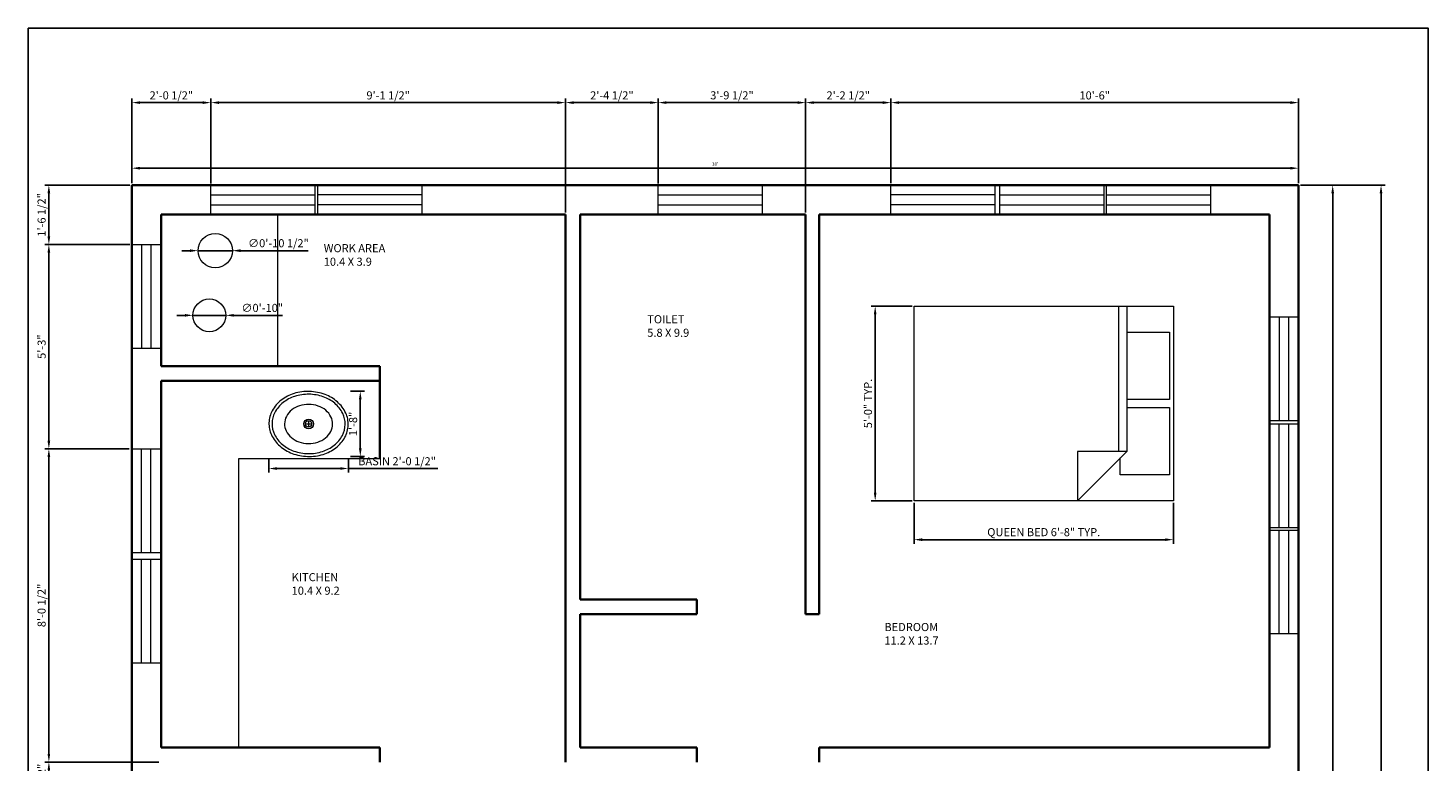
# Model space of a CAD drawing. Units: inches. Extents: x 185 to 617, y 27 to 601.
# Tile 2 of 2: x 185 to 617, y 374 to 601. Entities that reach past the tile are written whole.
import ezdxf

# ---------------------------------------------------------------- set-up
doc = ezdxf.new("R2010")
doc.units = ezdxf.units.IN
for name, color, linetype, lineweight in [('A-ANNO-DIMS', 2, 'Continuous', 18), ('A-ANNO-TTLB', 7, 'Continuous', 25), ('A-AREA-IDEN', 7, 'Continuous', 18), ('A-FLOR-FIXT', 9, 'Continuous', 18), ('A-FURN', 8, 'Continuous', 18), ('A-GLAZ', 4, 'Continuous', 18), ('A-WALL', 7, 'Continuous', 35)]:
    doc.layers.add(name, color=color, linetype=linetype, lineweight=lineweight)
doc.styles.get("Standard").update_dxf_attribs({"font": 'arial.ttf'})
doc.dimstyles.new('ISO-25', dxfattribs={"dimtxt": 2.5, "dimasz": 2.5, "dimexe": 1.25, "dimexo": 0.625, "dimtad": 1, "dimtxsty": 'Standard', "dimcen": 2.5, "dimadec": 0, "dimazin": 0, "dimtfac": 1, "dimtmove": 0, "dimatfit": 3, "dimfxl": 1, "dimarcsym": 0})

# ---------------------------------------------------------------- blocks, each defined once
blk = doc.blocks.new('Sink - Oval top')
for p, q in [((-1, 0), (1, 0)), ((0, 1), (0, -1))]:
    blk.add_line(p, q)
for points in [[(-12.23, 0.39, 0.117634), (-11.46, -3.36, 0.104469), (-8.88, -6.8, 0.090016), (-5.08, -9.07, 0.08192), (-0.32, -10.02, 0.08192), (4.49, -9.38, 0.090016), (8.42, -7.36, 0.104469), (11.22, -4.09, 0.117634), (12.23, -0.39, 0.117634), (11.46, 3.36, 0.104469), (8.88, 6.8, 0.090016), (5.08, 9.07, 0.08192), (0.32, 10.02, 0.08192), (-4.49, 9.38, 0.090016), (-8.42, 7.36, 0.104469), (-11.22, 4.09, 0.117634)], [(-11.29, 0.16, 0.118622), (-10.52, -3.25, 0.104678), (-8.07, -6.36, 0.089562), (-4.54, -8.37, 0.081185), (-0.13, -9.15, 0.081185), (4.3, -8.49, 0.089562), (7.89, -6.58, 0.104678), (10.42, -3.55, 0.118622), (11.29, -0.16, 0.118622), (10.52, 3.25, 0.104678), (8.07, 6.36, 0.089562), (4.54, 8.37, 0.081185), (0.13, 9.15, 0.081185), (-4.3, 8.49, 0.089562), (-7.89, 6.58, 0.104678), (-10.42, 3.55, 0.118622)], [(-7.42, 0.08, 0.118283), (-6.91, -2.17, 0.104607), (-5.29, -4.21, 0.089718), (-2.97, -5.53, 0.081436), (-0.07, -6.04, 0.081436), (2.84, -5.59, 0.089718), (5.2, -4.33, 0.104607), (6.86, -2.32, 0.118283), (7.42, -0.08, 0.118283), (6.91, 2.17, 0.104607), (5.29, 4.21, 0.089718), (2.97, 5.53, 0.081436), (0.07, 6.04, 0.081436), (-2.84, 5.59, 0.089718), (-5.2, 4.33, 0.104607), (-6.86, 2.32, 0.118283)]]:
    blk.add_lwpolyline(points, format="xyb", close=True)
for radius in [1.5, 1]:
    blk.add_circle((0, 0), radius)
blk = doc.blocks.new('Bed - Queen')
for p, q in [((0, -80.00003), (0, 0)), ((0, 0), (59.99999, 0)), ((59.99999, 0), (59.99999, -80.00003)), ((7.99999, -1.2), (28.79998, -1.2)), ((7.99999, -14.4), (7.99999, -1.2)), ((28.79998, -1.2), (28.79998, -14.4)), ((31.19999, -1.2), (51.99999, -1.2)), ((31.19999, -14.4), (31.19999, -1.2)), ((51.99999, -1.2), (51.99999, -16.4)), ((0, -14.4), (44.8, -14.4)), ((44.8, -16.8), (0, -16.8)), ((59.99999, -29.6), (44.8, -14.4)), ((44.8, -14.4), (44.8, -29.6)), ((51.99999, -16.4), (46.79936, -16.4)), ((44.8, -29.6), (59.99999, -29.6)), ((59.99999, -80.00003), (0, -80.00003))]:
    blk.add_line(p, q)
blk = doc.blocks.new('*D6')
at = {"layer": 'A-ANNO-DIMS', "color": 0, "lineweight": -2, "transparency": 16777216}
for p, q in [((217.11, 552.94), (217.11, 558.81)), ((219.61, 557.56), (574.61, 557.56)), ((577.11, 552.94), (577.11, 558.81))]:
    blk.add_line(p, q, dxfattribs=at)
at = {"layer": 'A-ANNO-DIMS', "color": 0, "transparency": 16777216}
for points in [[(219.61, 557.98), (219.61, 557.15), (217.11, 557.56)], [(574.61, 557.98), (574.61, 557.15), (577.11, 557.56)]]:
    blk.add_solid(points, dxfattribs=at)
at = {"layer": 'Defpoints', "color": 0, "transparency": 16777216}
for p in [(577.11, 557.56), (217.11, 552.31), (577.11, 552.31)]:
    blk.add_point(p, dxfattribs=at)
at = {"layer": 'A-ANNO-DIMS', "color": 0, "transparency": 16777216, "insert": (397.11, 558.7), "char_height": 1, "attachment_point": 5}
blk.add_mtext("30'", dxfattribs=at)
blk = doc.blocks.new('*D7')
at = {"layer": 'A-ANNO-DIMS', "color": 0, "lineweight": -2, "transparency": 16777216}
for p, q in [((577.73, 552.31), (588.89, 552.31)), ((587.64, 549.81), (587.64, 74.81)), ((577.73, 72.31), (588.89, 72.31))]:
    blk.add_line(p, q, dxfattribs=at)
at = {"layer": 'A-ANNO-DIMS', "color": 0, "transparency": 16777216}
for points in [[(587.22, 549.81), (588.05, 549.81), (587.64, 552.31)], [(587.22, 74.81), (588.05, 74.81), (587.64, 72.31)]]:
    blk.add_solid(points, dxfattribs=at)
at = {"layer": 'Defpoints', "color": 0, "transparency": 16777216}
for p in [(577.11, 552.31), (577.11, 72.31), (587.64, 72.31)]:
    blk.add_point(p, dxfattribs=at)
at = {"layer": 'A-ANNO-DIMS', "color": 0, "transparency": 16777216, "insert": (586.5, 312.31), "char_height": 1, "attachment_point": 5, "rotation": 90}
blk.add_mtext("40'", dxfattribs=at)
blk = doc.blocks.new('WIN-32IN-EXT')
for p, q in [((0, 0), (0, 32.06)), ((0, 32.06), (9, 32.06)), ((3, 32.06), (3, 0)), ((6, 0), (6, 32.06)), ((9, 32.06), (9, 0)), ((9, 0), (0, 0))]:
    blk.add_line(p, q)
blk = doc.blocks.new('*D19')
at = {"layer": 'A-ANNO-DIMS', "color": 0, "lineweight": -2, "transparency": 16777216}
for p, q in [((458.47, 454.36), (458.47, 441.73)), ((538.47, 454.36), (538.47, 441.73)), ((460.97, 442.98), (535.97, 442.98))]:
    blk.add_line(p, q, dxfattribs=at)
at = {"layer": 'A-ANNO-DIMS', "color": 0, "transparency": 16777216}
for points in [[(460.97, 443.4), (460.97, 442.57), (458.47, 442.98)], [(535.97, 443.4), (535.97, 442.57), (538.47, 442.98)]]:
    blk.add_solid(points, dxfattribs=at)
at = {"layer": 'Defpoints', "color": 0, "transparency": 16777216}
for p in [(458.47, 454.98), (538.47, 454.98), (538.47, 442.98)]:
    blk.add_point(p, dxfattribs=at)
at = {"layer": 'A-ANNO-DIMS', "color": 0, "transparency": 16777216, "insert": (498.47, 444.98), "char_height": 2.5, "attachment_point": 5}
blk.add_mtext('QUEEN BED 6\'-8" TYP.', dxfattribs=at)
blk = doc.blocks.new('*D20')
at = {"layer": 'A-ANNO-DIMS', "color": 0, "lineweight": -2, "transparency": 16777216}
for p, q in [((457.84, 514.98), (445.22, 514.98)), ((446.47, 512.48), (446.47, 457.48)), ((457.84, 454.98), (445.22, 454.98))]:
    blk.add_line(p, q, dxfattribs=at)
at = {"layer": 'A-ANNO-DIMS', "color": 0, "transparency": 16777216}
for points in [[(446.05, 512.48), (446.88, 512.48), (446.47, 514.98)], [(446.05, 457.48), (446.88, 457.48), (446.47, 454.98)]]:
    blk.add_solid(points, dxfattribs=at)
at = {"layer": 'Defpoints', "color": 0, "transparency": 16777216}
for p in [(458.47, 514.98), (446.47, 454.98), (458.47, 454.98)]:
    blk.add_point(p, dxfattribs=at)
at = {"layer": 'A-ANNO-DIMS', "color": 0, "transparency": 16777216, "insert": (444.57, 484.98), "char_height": 2.5, "attachment_point": 5, "rotation": 90}
blk.add_mtext('5\'-0" TYP.', dxfattribs=at)
blk = doc.blocks.new('*D23')
at = {"layer": 'A-ANNO-DIMS', "color": 0, "lineweight": -2, "transparency": 16777216}
for p, q in [((259.36, 467.99), (259.36, 463.68)), ((283.91, 467.99), (283.91, 463.68)), ((261.86, 464.93), (281.41, 464.93)), ((283.91, 464.93), (311.47, 464.93))]:
    blk.add_line(p, q, dxfattribs=at)
at = {"layer": 'A-ANNO-DIMS', "color": 0, "transparency": 16777216}
for points in [[(261.86, 465.35), (261.86, 464.52), (259.36, 464.93)], [(281.41, 465.35), (281.41, 464.52), (283.91, 464.93)]]:
    blk.add_solid(points, dxfattribs=at)
at = {"layer": 'Defpoints', "color": 0, "transparency": 16777216}
for p in [(259.36, 468.62), (283.91, 468.62), (283.91, 464.93)]:
    blk.add_point(p, dxfattribs=at)
at = {"layer": 'A-ANNO-DIMS', "color": 0, "transparency": 16777216, "insert": (298.94, 466.85), "char_height": 2.5, "attachment_point": 5}
blk.add_mtext('BASIN 2\'-0 1/2"', dxfattribs=at)
blk = doc.blocks.new('*D24')
at = {"layer": 'A-ANNO-DIMS', "color": 0, "lineweight": -2, "transparency": 16777216}
for p, q in [((284.54, 488.75), (288.84, 488.75)), ((287.59, 471.12), (287.59, 486.25)), ((284.54, 468.62), (288.84, 468.62))]:
    blk.add_line(p, q, dxfattribs=at)
at = {"layer": 'A-ANNO-DIMS', "color": 0, "transparency": 16777216}
for points in [[(287.18, 486.25), (288.01, 486.25), (287.59, 488.75)], [(287.18, 471.12), (288.01, 471.12), (287.59, 468.62)]]:
    blk.add_solid(points, dxfattribs=at)
at = {"layer": 'Defpoints', "color": 0, "transparency": 16777216}
for p in [(283.91, 488.75), (287.59, 488.75), (283.91, 468.62)]:
    blk.add_point(p, dxfattribs=at)
at = {"layer": 'A-ANNO-DIMS', "color": 0, "transparency": 16777216, "insert": (285.69, 478.68), "char_height": 2.5, "attachment_point": 5, "rotation": 90}
blk.add_mtext('1\'-8"', dxfattribs=at)
blk = doc.blocks.new('*D25')
at = {"layer": 'A-ANNO-DIMS', "color": 0, "lineweight": -2, "transparency": 16777216}
for p, q in [((577.73, 552.31), (603.81, 552.31)), ((602.56, 63.07), (602.56, 549.81)), ((429.78, 60.57), (603.81, 60.57))]:
    blk.add_line(p, q, dxfattribs=at)
at = {"layer": 'A-ANNO-DIMS', "color": 0, "transparency": 16777216}
for points in [[(602.14, 549.81), (602.97, 549.81), (602.56, 552.31)], [(602.14, 63.07), (602.97, 63.07), (602.56, 60.57)]]:
    blk.add_solid(points, dxfattribs=at)
at = {"layer": 'Defpoints', "color": 0, "transparency": 16777216}
for p in [(577.11, 552.31), (602.56, 552.31), (429.16, 60.57)]:
    blk.add_point(p, dxfattribs=at)
at = {"layer": 'A-ANNO-DIMS', "color": 0, "transparency": 16777216, "insert": (600.64, 306.44), "char_height": 2.5, "attachment_point": 5, "rotation": 90}
blk.add_mtext('40\'-11 1/2"', dxfattribs=at)
blk = doc.blocks.new('*D31')
at = {"layer": 'A-ANNO-DIMS', "color": 0, "lineweight": -2, "transparency": 16777216}
for p, q in [((217.11, 552.94), (217.11, 579.04)), ((241.48, 552.86), (241.48, 579.04)), ((219.61, 577.79), (238.98, 577.79))]:
    blk.add_line(p, q, dxfattribs=at)
at = {"layer": 'A-ANNO-DIMS', "color": 0, "transparency": 16777216}
for points in [[(219.61, 578.2), (219.61, 577.37), (217.11, 577.79)], [(238.98, 578.2), (238.98, 577.37), (241.48, 577.79)]]:
    blk.add_solid(points, dxfattribs=at)
at = {"layer": 'Defpoints', "color": 0, "transparency": 16777216}
for p in [(241.48, 577.79), (217.11, 552.31), (241.48, 552.23)]:
    blk.add_point(p, dxfattribs=at)
at = {"layer": 'A-ANNO-DIMS', "color": 0, "transparency": 16777216, "insert": (229.29, 579.7), "char_height": 2.5, "attachment_point": 5}
blk.add_mtext('2\'-0 1/2"', dxfattribs=at)
blk = doc.blocks.new('*D32')
at = {"layer": 'A-ANNO-DIMS', "color": 0, "lineweight": -2, "transparency": 16777216}
for p, q in [((241.48, 552.86), (241.48, 579.04)), ((350.91, 543.94), (350.91, 579.04)), ((243.98, 577.79), (348.41, 577.79))]:
    blk.add_line(p, q, dxfattribs=at)
at = {"layer": 'A-ANNO-DIMS', "color": 0, "transparency": 16777216}
for points in [[(243.98, 578.2), (243.98, 577.37), (241.48, 577.79)], [(348.41, 578.2), (348.41, 577.37), (350.91, 577.79)]]:
    blk.add_solid(points, dxfattribs=at)
at = {"layer": 'Defpoints', "color": 0, "transparency": 16777216}
for p in [(350.91, 577.79), (241.48, 552.23), (350.91, 543.31)]:
    blk.add_point(p, dxfattribs=at)
at = {"layer": 'A-ANNO-DIMS', "color": 0, "transparency": 16777216, "insert": (296.19, 579.7), "char_height": 2.5, "attachment_point": 5}
blk.add_mtext('9\'-1 1/2"', dxfattribs=at)
blk = doc.blocks.new('*D33')
at = {"layer": 'A-ANNO-DIMS', "color": 0, "lineweight": -2, "transparency": 16777216}
for p, q in [((350.91, 543.94), (350.91, 579.04)), ((379.55, 552.85), (379.55, 579.04)), ((353.41, 577.79), (377.05, 577.79))]:
    blk.add_line(p, q, dxfattribs=at)
at = {"layer": 'A-ANNO-DIMS', "color": 0, "transparency": 16777216}
for points in [[(353.41, 578.2), (353.41, 577.37), (350.91, 577.79)], [(377.05, 578.2), (377.05, 577.37), (379.55, 577.79)]]:
    blk.add_solid(points, dxfattribs=at)
at = {"layer": 'Defpoints', "color": 0, "transparency": 16777216}
for p in [(379.55, 577.79), (379.55, 552.22), (350.91, 543.31)]:
    blk.add_point(p, dxfattribs=at)
at = {"layer": 'A-ANNO-DIMS', "color": 0, "transparency": 16777216, "insert": (365.23, 579.7), "char_height": 2.5, "attachment_point": 5}
blk.add_mtext('2\'-4 1/2"', dxfattribs=at)
blk = doc.blocks.new('*D34')
at = {"layer": 'A-ANNO-DIMS', "color": 0, "lineweight": -2, "transparency": 16777216}
for p, q in [((379.55, 552.85), (379.55, 579.04)), ((425.01, 543.94), (425.01, 579.04)), ((382.05, 577.79), (422.51, 577.79))]:
    blk.add_line(p, q, dxfattribs=at)
at = {"layer": 'A-ANNO-DIMS', "color": 0, "transparency": 16777216}
for points in [[(382.05, 578.2), (382.05, 577.37), (379.55, 577.79)], [(422.51, 578.2), (422.51, 577.37), (425.01, 577.79)]]:
    blk.add_solid(points, dxfattribs=at)
at = {"layer": 'Defpoints', "color": 0, "transparency": 16777216}
for p in [(425.01, 577.79), (379.55, 552.22), (425.01, 543.31)]:
    blk.add_point(p, dxfattribs=at)
at = {"layer": 'A-ANNO-DIMS', "color": 0, "transparency": 16777216, "insert": (402.28, 579.71), "char_height": 2.5, "attachment_point": 5}
blk.add_mtext('3\'-9 1/2"', dxfattribs=at)
blk = doc.blocks.new('*D35')
at = {"layer": 'A-ANNO-DIMS', "color": 0, "lineweight": -2, "transparency": 16777216}
for p, q in [((425.01, 543.94), (425.01, 579.04)), ((451.32, 552.96), (451.32, 579.04)), ((427.51, 577.79), (448.82, 577.79))]:
    blk.add_line(p, q, dxfattribs=at)
at = {"layer": 'A-ANNO-DIMS', "color": 0, "transparency": 16777216}
for points in [[(427.51, 578.2), (427.51, 577.37), (425.01, 577.79)], [(448.82, 578.2), (448.82, 577.37), (451.32, 577.79)]]:
    blk.add_solid(points, dxfattribs=at)
at = {"layer": 'Defpoints', "color": 0, "transparency": 16777216}
for p in [(451.32, 577.79), (451.32, 552.34), (425.01, 543.31)]:
    blk.add_point(p, dxfattribs=at)
at = {"layer": 'A-ANNO-DIMS', "color": 0, "transparency": 16777216, "insert": (438.16, 579.7), "char_height": 2.5, "attachment_point": 5}
blk.add_mtext('2\'-2 1/2"', dxfattribs=at)
blk = doc.blocks.new('*D36')
at = {"layer": 'A-ANNO-DIMS', "color": 0, "lineweight": -2, "transparency": 16777216}
for p, q in [((451.32, 552.96), (451.32, 579.04)), ((577.11, 552.94), (577.11, 579.04)), ((453.82, 577.79), (574.61, 577.79))]:
    blk.add_line(p, q, dxfattribs=at)
at = {"layer": 'A-ANNO-DIMS', "color": 0, "transparency": 16777216}
for points in [[(453.82, 578.2), (453.82, 577.37), (451.32, 577.79)], [(574.61, 578.2), (574.61, 577.37), (577.11, 577.79)]]:
    blk.add_solid(points, dxfattribs=at)
at = {"layer": 'Defpoints', "color": 0, "transparency": 16777216}
for p in [(577.11, 577.79), (451.32, 552.34), (577.11, 552.31)]:
    blk.add_point(p, dxfattribs=at)
at = {"layer": 'A-ANNO-DIMS', "color": 0, "transparency": 16777216, "insert": (514.21, 579.69), "char_height": 2.5, "attachment_point": 5}
blk.add_mtext('10\'-6"', dxfattribs=at)
blk = doc.blocks.new('*D37')
at = {"layer": 'A-ANNO-DIMS', "color": 0, "lineweight": -2, "transparency": 16777216}
for p, q in [((216.48, 552.31), (190.25, 552.31)), ((191.5, 549.81), (191.5, 536.5)), ((216.46, 534), (190.25, 534))]:
    blk.add_line(p, q, dxfattribs=at)
at = {"layer": 'A-ANNO-DIMS', "color": 0, "transparency": 16777216}
for points in [[(191.08, 549.81), (191.91, 549.81), (191.5, 552.31)], [(191.08, 536.5), (191.91, 536.5), (191.5, 534)]]:
    blk.add_solid(points, dxfattribs=at)
at = {"layer": 'Defpoints', "color": 0, "transparency": 16777216}
for p in [(217.11, 552.31), (191.5, 534), (217.08, 534)]:
    blk.add_point(p, dxfattribs=at)
at = {"layer": 'A-ANNO-DIMS', "color": 0, "transparency": 16777216, "insert": (189.58, 543.16), "char_height": 2.5, "attachment_point": 5, "rotation": 90}
blk.add_mtext('1\'-6 1/2"', dxfattribs=at)
blk = doc.blocks.new('*D38')
at = {"layer": 'A-ANNO-DIMS', "color": 0, "lineweight": -2, "transparency": 16777216}
for p, q in [((216.46, 534), (190.25, 534)), ((191.5, 531.5), (191.5, 473.52)), ((216.32, 471.02), (190.25, 471.02))]:
    blk.add_line(p, q, dxfattribs=at)
at = {"layer": 'A-ANNO-DIMS', "color": 0, "transparency": 16777216}
for points in [[(191.08, 531.5), (191.91, 531.5), (191.5, 534)], [(191.08, 473.52), (191.91, 473.52), (191.5, 471.02)]]:
    blk.add_solid(points, dxfattribs=at)
at = {"layer": 'Defpoints', "color": 0, "transparency": 16777216}
for p in [(217.08, 534), (191.5, 471.02), (216.95, 471.02)]:
    blk.add_point(p, dxfattribs=at)
at = {"layer": 'A-ANNO-DIMS', "color": 0, "transparency": 16777216, "insert": (189.59, 502.51), "char_height": 2.5, "attachment_point": 5, "rotation": 90}
blk.add_mtext('5\'-3"', dxfattribs=at)
blk = doc.blocks.new('*D39')
at = {"layer": 'A-ANNO-DIMS', "color": 0, "lineweight": -2, "transparency": 16777216}
for p, q in [((216.32, 471.02), (190.25, 471.02)), ((191.5, 468.52), (191.5, 376.91)), ((225.48, 374.41), (190.25, 374.41))]:
    blk.add_line(p, q, dxfattribs=at)
at = {"layer": 'A-ANNO-DIMS', "color": 0, "transparency": 16777216}
for points in [[(191.08, 468.52), (191.91, 468.52), (191.5, 471.02)], [(191.08, 376.91), (191.91, 376.91), (191.5, 374.41)]]:
    blk.add_solid(points, dxfattribs=at)
at = {"layer": 'Defpoints', "color": 0, "transparency": 16777216}
for p in [(216.95, 471.02), (191.5, 374.41), (226.11, 374.41)]:
    blk.add_point(p, dxfattribs=at)
at = {"layer": 'A-ANNO-DIMS', "color": 0, "transparency": 16777216, "insert": (189.58, 422.71), "char_height": 2.5, "attachment_point": 5, "rotation": 90}
blk.add_mtext('8\'-0 1/2"', dxfattribs=at)
blk = doc.blocks.new('*D40')
at = {"layer": 'A-ANNO-DIMS', "color": 0, "lineweight": -2, "transparency": 16777216}
for p, q in [((225.48, 374.41), (190.25, 374.41)), ((191.5, 371.91), (191.5, 362.42)), ((216.42, 359.92), (190.25, 359.92))]:
    blk.add_line(p, q, dxfattribs=at)
at = {"layer": 'A-ANNO-DIMS', "color": 0, "transparency": 16777216}
for points in [[(191.08, 371.91), (191.91, 371.91), (191.5, 374.41)], [(191.08, 362.42), (191.91, 362.42), (191.5, 359.92)]]:
    blk.add_solid(points, dxfattribs=at)
at = {"layer": 'Defpoints', "color": 0, "transparency": 16777216}
for p in [(226.11, 374.41), (191.5, 359.92), (217.05, 359.92)]:
    blk.add_point(p, dxfattribs=at)
at = {"layer": 'A-ANNO-DIMS', "color": 0, "transparency": 16777216, "insert": (189.58, 367.17), "char_height": 2.5, "attachment_point": 5, "rotation": 90}
blk.add_mtext('1\'-2 1/2"', dxfattribs=at)
blk = doc.blocks.new('*D44')
at = {"layer": 'A-ANNO-DIMS', "color": 0, "lineweight": -2, "transparency": 16777216}
for p, q in [((235.02, 532.12), (232.52, 532.12)), ((237.52, 532.12), (248.14, 532.12)), ((271.52, 532.12), (250.64, 532.12))]:
    blk.add_line(p, q, dxfattribs=at)
at = {"layer": 'A-ANNO-DIMS', "color": 0, "transparency": 16777216}
for points in [[(235.02, 532.54), (235.02, 531.71), (237.52, 532.12)], [(250.64, 532.54), (250.64, 531.71), (248.14, 532.12)]]:
    blk.add_solid(points, dxfattribs=at)
at = {"layer": 'Defpoints', "color": 0, "transparency": 16777216}
for p in [(237.52, 532.12), (248.14, 532.12)]:
    blk.add_point(p, dxfattribs=at)
at = {"layer": 'A-ANNO-DIMS', "color": 0, "transparency": 16777216, "insert": (262.33, 534.1), "char_height": 2.5, "attachment_point": 5, "rotation": 0.0037}
blk.add_mtext('∅0\'-10 1/2"', dxfattribs=at)
blk = doc.blocks.new('*D45')
at = {"layer": 'A-ANNO-DIMS', "color": 0, "lineweight": -2, "transparency": 16777216}
for p, q in [((233.46, 512.17), (230.96, 512.17)), ((235.96, 512.17), (246.07, 512.17)), ((263.62, 512.17), (248.57, 512.17))]:
    blk.add_line(p, q, dxfattribs=at)
at = {"layer": 'A-ANNO-DIMS', "color": 0, "transparency": 16777216}
for points in [[(233.46, 512.59), (233.46, 511.75), (235.96, 512.17)], [(248.57, 512.59), (248.57, 511.76), (246.07, 512.17)]]:
    blk.add_solid(points, dxfattribs=at)
at = {"layer": 'Defpoints', "color": 0, "transparency": 16777216}
for p in [(235.96, 512.17), (246.07, 512.17)]:
    blk.add_point(p, dxfattribs=at)
at = {"layer": 'A-ANNO-DIMS', "color": 0, "transparency": 16777216, "insert": (257.34, 514.14), "char_height": 2.5, "attachment_point": 5, "rotation": 0.0054}
blk.add_mtext('∅0\'-10"', dxfattribs=at)

msp = doc.modelspace()

# ---------------------------------------------------------------- linework, layer by layer
at = {"layer": 'A-ANNO-TTLB'}
msp.add_lwpolyline([(185.06, 600.8), (617.05, 600.8), (617.05, 26.91), (185.06, 26.91)], close=True, dxfattribs=at)
at = {"layer": 'A-FLOR-FIXT'}
for p, q in [((262.11, 496.51), (262.11, 543.31)), ((250.11, 468.01), (293.61, 468.01)), ((250.11, 378.91), (250.11, 468.01))]:
    msp.add_line(p, q, dxfattribs=at)
for centre, radius in [((242.83, 532.12), 5.31), ((241.01, 512.17), 5.05)]:
    msp.add_circle(centre, radius, dxfattribs=at)
at = {"layer": 'A-WALL'}
for p, q in [((217.11, 72.31), (217.11, 552.31)), ((217.11, 552.31), (577.11, 552.31)), ((577.11, 552.31), (577.11, 72.31)), ((226.11, 543.31), (350.91, 543.31)), ((226.11, 496.51), (226.11, 543.31)), ((350.91, 374.41), (350.91, 543.31)), ((350.91, 374.41), (350.91, 543.31)), ((355.41, 424.51), (355.41, 543.31)), ((355.41, 543.31), (425.01, 543.31)), ((425.01, 420.01), (425.01, 543.31)), ((429.21, 543.31), (429.21, 420.01)), ((429.21, 543.31), (568.11, 543.31)), ((568.11, 543.31), (568.11, 378.91)), ((226.11, 496.51), (293.61, 496.51)), ((293.61, 496.51), (293.61, 468.01)), ((226.11, 492.01), (293.61, 492.01)), ((226.11, 378.91), (226.11, 492.01)), ((355.41, 424.51), (391.41, 424.51)), ((391.41, 420.01), (391.41, 424.51)), ((355.41, 420.01), (391.41, 420.01)), ((355.41, 378.91), (355.41, 420.01)), ((425.01, 420.01), (429.21, 420.01)), ((226.11, 378.91), (293.61, 378.91)), ((293.61, 378.91), (293.61, 374.41)), ((355.41, 378.91), (391.41, 378.91)), ((391.41, 374.41), (391.41, 378.91)), ((429.21, 378.91), (429.21, 374.41)), ((429.21, 378.91), (433.71, 378.91)), ((433.71, 378.91), (568.11, 378.91))]:
    msp.add_line(p, q, dxfattribs=at)

# ---------------------------------------------------------------- block references
at = {"layer": 'A-FLOR-FIXT'}
msp.add_blockref('Sink - Oval top', (271.64, 478.68), dxfattribs=at)
at = {"layer": 'A-FURN', "rotation": 270}
msp.add_blockref('Bed - Queen', (538.47, 514.98), dxfattribs=at)
at = {"layer": 'A-GLAZ'}
for p, rotation in [((241.48, 552.23), 270), ((274.53, 552.32), 270.0000000000001), ((379.55, 552.22), 270.0000000000001), ((451.32, 552.34), 270.0000000000001), ((484.92, 552.25), 269.9999999999998), ((517.89, 552.25), 269.9999999999997), ((226.08, 534), 180), ((577.1, 511.71), 180), ((577.07, 478.7), 180), ((225.95, 471.01), 180), ((577.06, 445.96), 180), ((225.95, 436.96), 180)]:
    msp.add_blockref('WIN-32IN-EXT', p, dxfattribs=dict(at, rotation=rotation))

# ---------------------------------------------------------------- texts
at = {"layer": 'A-AREA-IDEN', "char_height": 2.5, "attachment_point": 1}
for s, width, insert in [('WORK AREA\\P10.4 X 3.9', 44.1813, (276.32, 534.14)), ('TOILET\\P5.8 X 9.9', 49.908, (376.14, 512.22)), ('KITCHEN\\P10.4 X 9.2', 44.0935, (266.41, 432.67)), ('BEDROOM\\P11.2 X 13.7', 62.5607, (449.31, 417.29))]:
    msp.add_mtext_dynamic_manual_height_columns(s, width=width, gutter_width=12.5, heights=[0], dxfattribs=dict(at, insert=insert))

# ---------------------------------------------------------------- dimensions: what is measured, and where the dimension line sits
at = {"layer": 'A-ANNO-DIMS'}
for base, p1, p2, override, picture, middle in [((241.48, 577.79), (217.11, 552.31), (241.48, 552.23), {"dimdec": 1, "dimlfac": 1, "dimrnd": 0, "dimzin": 1, "dimdsep": 46, "dimlunit": 4, "dimfrac": 2}, '*D31', (229.29, 579.7)), ((350.91, 577.79), (241.48, 552.23), (350.91, 543.31), {"dimdec": 1, "dimlfac": 1, "dimrnd": 0, "dimzin": 1, "dimdsep": 46, "dimlunit": 4, "dimfrac": 2}, '*D32', (296.19, 579.7)), ((379.55, 577.79), (350.91, 543.31), (379.55, 552.22), {"dimdec": 1, "dimlfac": 1, "dimrnd": 0, "dimzin": 1, "dimdsep": 46, "dimlunit": 4, "dimfrac": 2}, '*D33', (365.23, 579.7)), ((425.01, 577.79), (379.55, 552.22), (425.01, 543.31), {"dimdec": 1, "dimlfac": 1, "dimrnd": 0, "dimzin": 1, "dimdsep": 46, "dimlunit": 4, "dimfrac": 2}, '*D34', (402.28, 579.71)), ((451.32, 577.79), (425.01, 543.31), (451.32, 552.34), {"dimdec": 1, "dimlfac": 1, "dimrnd": 0, "dimzin": 1, "dimdsep": 46, "dimlunit": 4, "dimfrac": 2}, '*D35', (438.16, 579.7)), ((577.11, 577.79), (451.32, 552.34), (577.11, 552.31), {"dimdec": 1, "dimlfac": 1, "dimrnd": 0, "dimzin": 1, "dimdsep": 46, "dimlunit": 4, "dimfrac": 2}, '*D36', (514.21, 579.69)), ((577.11, 557.56), (217.11, 552.31), (577.11, 552.31), {"dimtxt": 1, "dimdec": 0, "dimlunit": 3, "dimclrd": 0, "dimclre": 0, "dimclrt": 0, "dimtdec": 0}, '*D6', (397.11, 558.7))]:
    dim = msp.add_linear_dim(base=base, p1=p1, p2=p2, dimstyle='ISO-25', override=override, dxfattribs=at)
    dim.commit()
    dim.dimension.update_dxf_attribs({"geometry": picture, "text_midpoint": middle})
for base, p1, p2, override, picture, middle in [((191.5, 534), (217.11, 552.31), (217.08, 534), {"dimdec": 1, "dimlfac": 1, "dimrnd": 0, "dimzin": 1, "dimdsep": 46, "dimlunit": 4, "dimfrac": 2}, '*D37', (189.58, 543.16)), ((602.56, 552.31), (429.16, 60.57), (577.11, 552.31), {"dimdec": 1, "dimlfac": 1, "dimrnd": 0, "dimzin": 1, "dimdsep": 46, "dimlunit": 4, "dimfrac": 2}, '*D25', (600.64, 306.44)), ((587.64, 72.31), (577.11, 552.31), (577.11, 72.31), {"dimtxt": 1, "dimdec": 0, "dimlunit": 3, "dimclrd": 0, "dimclre": 0, "dimclrt": 0, "dimtdec": 0}, '*D7', (586.5, 312.31)), ((191.5, 471.02), (217.08, 534), (216.95, 471.02), {"dimdec": 1, "dimlfac": 1, "dimrnd": 0, "dimzin": 1, "dimdsep": 46, "dimlunit": 4, "dimfrac": 2}, '*D38', (189.59, 502.51)), ((287.59, 488.75), (283.91, 468.62), (283.91, 488.75), {"dimdec": 1, "dimlfac": 1, "dimrnd": 0, "dimzin": 1, "dimdsep": 46, "dimlunit": 4, "dimfrac": 2}, '*D24', (285.69, 478.68)), ((191.5, 374.41), (216.95, 471.02), (226.11, 374.41), {"dimdec": 1, "dimlfac": 1, "dimrnd": 0, "dimzin": 1, "dimdsep": 46, "dimlunit": 4, "dimfrac": 2}, '*D39', (189.58, 422.71)), ((191.5, 359.92), (226.11, 374.41), (217.05, 359.92), {"dimdec": 1, "dimlfac": 1, "dimrnd": 0, "dimzin": 1, "dimdsep": 46, "dimlunit": 4, "dimfrac": 2}, '*D40', (189.58, 367.17))]:
    dim = msp.add_linear_dim(base=base, p1=p1, p2=p2, angle=90, dimstyle='ISO-25', override=override, dxfattribs=at)
    dim.commit()
    dim.dimension.update_dxf_attribs({"geometry": picture, "text_midpoint": middle})
for p1, p2, picture, middle in [((237.52, 532.12), (248.14, 532.12), '*D44', (262.33, 532.12)), ((235.96, 512.17), (246.07, 512.17), '*D45', (257.35, 512.17))]:
    dim = msp.add_diameter_dim_2p(p1=p1, p2=p2, dimstyle='ISO-25', override={"dimdec": 1, "dimlfac": 1, "dimrnd": 0, "dimzin": 1, "dimdsep": 46, "dimlunit": 4, "dimfrac": 2}, dxfattribs=at)
    dim.commit()
    dim.dimension.update_dxf_attribs({"geometry": picture, "text_midpoint": middle})
dim = msp.add_linear_dim(base=(446.47, 454.98), p1=(458.47, 514.98), p2=(458.47, 454.98), angle=270, text='<> TYP.', dimstyle='ISO-25', override={"dimdec": 1, "dimlfac": 1, "dimrnd": 0, "dimzin": 1, "dimdsep": 46, "dimlunit": 4, "dimfrac": 2}, dxfattribs=at)
dim.commit()
dim.dimension.update_dxf_attribs({"geometry": '*D20', "text_midpoint": (444.57, 484.98)})
for base, p1, p2, text, picture, middle in [((283.9123, 464.9333), (259.3614, 468.6159), (283.9123, 468.6159), 'BASIN <>', '*D23', (298.943, 466.8509)), ((538.47, 442.98), (458.47, 454.98), (538.47, 454.98), 'QUEEN BED <> TYP.', '*D19', (498.47, 444.98))]:
    dim = msp.add_linear_dim(base=base, p1=p1, p2=p2, text=text, dimstyle='ISO-25', override={"dimdec": 1, "dimlfac": 1, "dimrnd": 0, "dimzin": 1, "dimdsep": 46, "dimlunit": 4, "dimfrac": 2}, dxfattribs=at)
    dim.commit()
    dim.dimension.update_dxf_attribs({"geometry": picture, "text_midpoint": middle})

doc.saveas('drawing.dxf')
